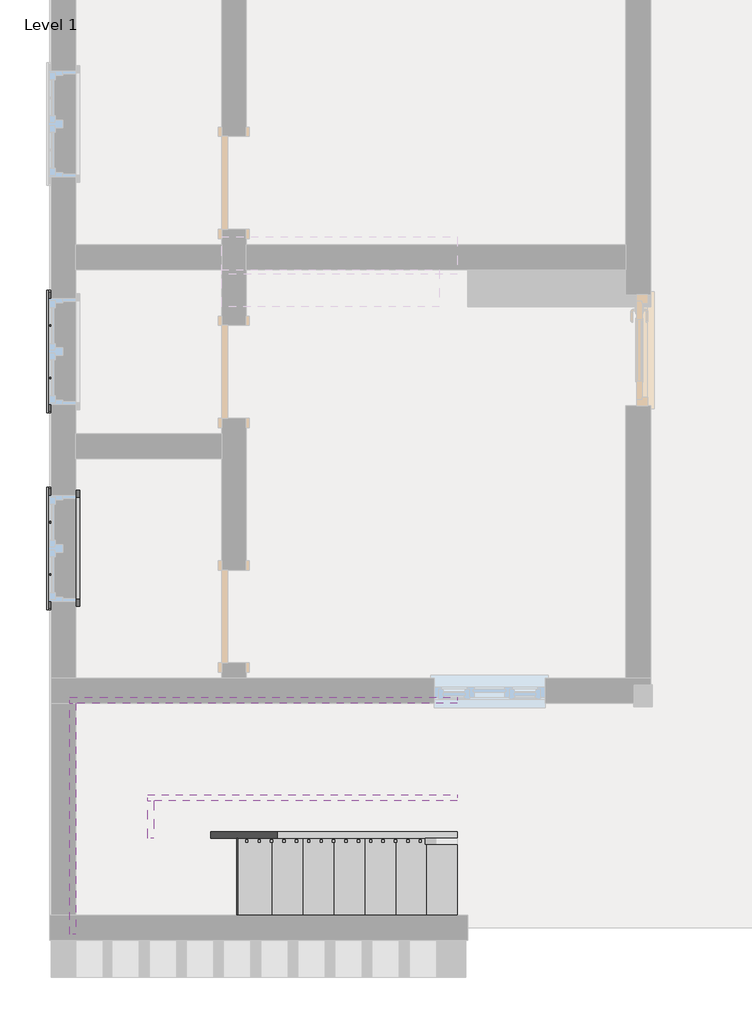
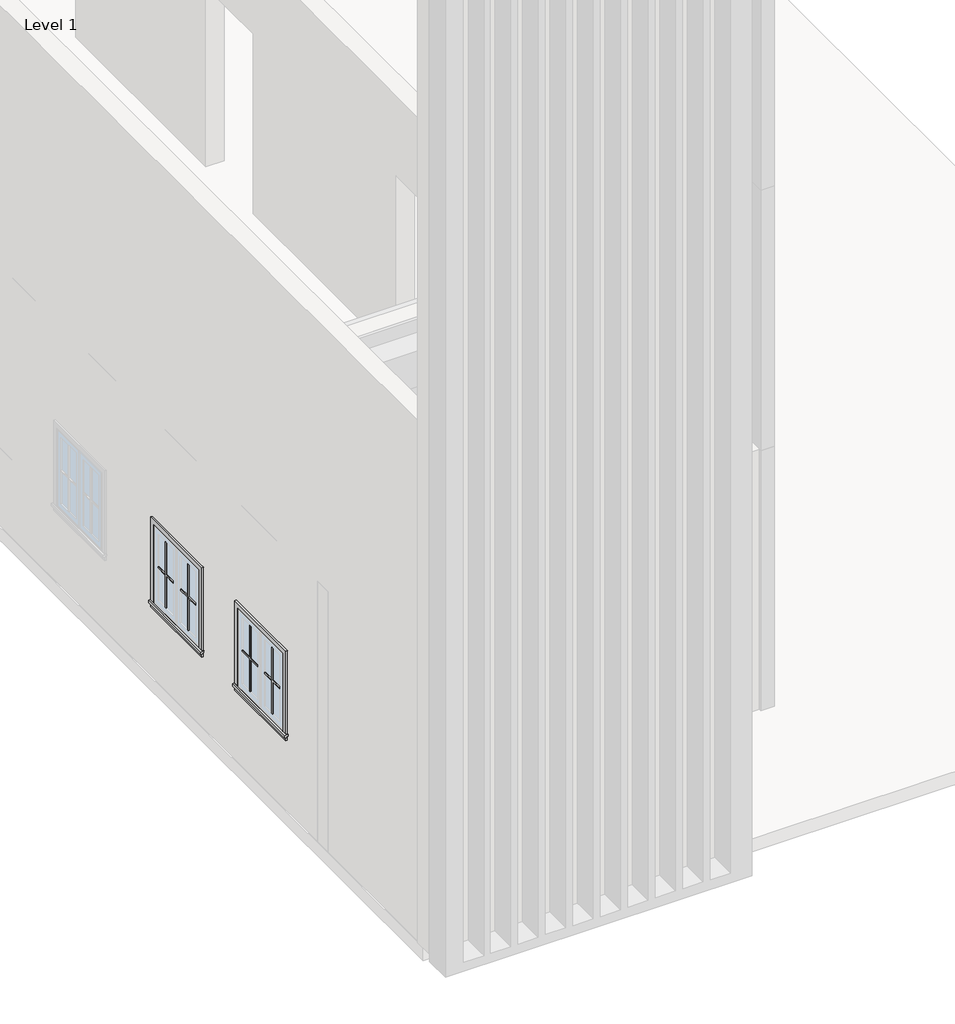
# One storey, part 3 of 4: 7 proxies, 6 members, 1 railing, 1 stair flight.
"""IFC4 building model written with IfcOpenShell, lengths in millimetres."""

from ifc_helpers import new_model, si_unit, frame, origin, place, context, project, spatial, polyline, outline, extrude, faceted_brep, transform, mapped, element, save
from components import muntin_pattern_2x2_muntin_pattern_2x2_b3fe6957, muntin_pattern_2x2_muntin_pattern_2x2_3e0ecaf2, trim_window_exterior_flat_with_sill_41619996, trim_window_interior_flat_picture_frame_51c85655, stair_flight_05893867

model = new_model("IFC4")

# Units and contexts
model_context = context("Model", 3, world=origin())
ifc_project = project(units=[si_unit("LENGTHUNIT", "METRE", prefix="MILLI")], contexts=[model_context])

# Site, building, storey
site = spatial("IfcSite", under=ifc_project)
building = spatial("IfcBuilding", under=site)
storey = spatial("IfcBuildingStorey", under=building, Name="Level 1", Elevation=0.0)

# Proxies
placement = place(None, origin())
muntin_pattern_2x2_muntin_pattern_2x2_shape = muntin_pattern_2x2_muntin_pattern_2x2_b3fe6957(model_context)
element("IfcBuildingElementProxy", 1, Name="Muntin Pattern_2x2 : Muntin Pattern_2x2", ObjectType="Muntin Pattern_2x2 : Muntin Pattern_2x2", at=placement, inside=storey, context=model_context, shape_type="MappedRepresentation", body=[
    mapped(muntin_pattern_2x2_muntin_pattern_2x2_shape, transform((-6438.8858866, -3658.1725272, 984.25), x_axis=(0.0, 1.0, 0.0), y_axis=(-1.0, 0.0, 0.0), z_axis=(0.0, 0.0, 1.0))),
])
element("IfcBuildingElementProxy", 2, Name="Muntin Pattern_2x2 : Muntin Pattern_2x2", ObjectType="Muntin Pattern_2x2 : Muntin Pattern_2x2", at=placement, inside=storey, context=model_context, shape_type="MappedRepresentation", body=[
    mapped(muntin_pattern_2x2_muntin_pattern_2x2_shape, transform((-6438.8858866, -5271.0725272, 984.25), x_axis=(0.0, 1.0, 0.0), y_axis=(-1.0, 0.0, 0.0), z_axis=(0.0, 0.0, 1.0))),
])
muntin_pattern_2x2_muntin_pattern_2x2_2_shape = muntin_pattern_2x2_muntin_pattern_2x2_3e0ecaf2(model_context)
element("IfcBuildingElementProxy", 3, Name="Muntin Pattern_2x2 : Muntin Pattern_2x2", ObjectType="Muntin Pattern_2x2 : Muntin Pattern_2x2", at=placement, inside=storey, context=model_context, shape_type="MappedRepresentation", body=[
    mapped(muntin_pattern_2x2_muntin_pattern_2x2_2_shape, transform((-6438.8858866, -3229.5475272, 984.25), x_axis=(0.0, -1.0, 0.0), y_axis=(1.0, 0.0, 0.0), z_axis=(0.0, 0.0, 1.0))),
])
element("IfcBuildingElementProxy", 4, Name="Muntin Pattern_2x2 : Muntin Pattern_2x2", ObjectType="Muntin Pattern_2x2 : Muntin Pattern_2x2", at=placement, inside=storey, context=model_context, shape_type="MappedRepresentation", body=[
    mapped(muntin_pattern_2x2_muntin_pattern_2x2_2_shape, transform((-6438.8858866, -4842.4475272, 984.25), x_axis=(0.0, -1.0, 0.0), y_axis=(1.0, 0.0, 0.0), z_axis=(0.0, 0.0, 1.0))),
])
trim_window_exterior_flat_with_sill_shape = trim_window_exterior_flat_with_sill_41619996(model_context)
element("IfcBuildingElementProxy", 5, Name="Trim-Window-Exterior-Flat : with Sill", ObjectType="Trim-Window-Exterior-Flat : with Sill", at=placement, inside=storey, context=model_context, shape_type="MappedRepresentation", body=[
    mapped(trim_window_exterior_flat_with_sill_shape, transform((-6448.4108866, -3443.8600272, 1828.8), x_axis=(0.0, -1.0, 0.0), y_axis=(0.0, 0.0, 1.0), z_axis=(-1.0, 0.0, 0.0))),
])
element("IfcBuildingElementProxy", 6, Name="Trim-Window-Exterior-Flat : with Sill", ObjectType="Trim-Window-Exterior-Flat : with Sill", at=placement, inside=storey, context=model_context, shape_type="MappedRepresentation", body=[
    mapped(trim_window_exterior_flat_with_sill_shape, transform((-6448.4108866, -5056.7600272, 1828.8), x_axis=(0.0, -1.0, 0.0), y_axis=(0.0, 0.0, 1.0), z_axis=(-1.0, 0.0, 0.0))),
])
trim_window_interior_flat_picture_frame_shape = trim_window_interior_flat_picture_frame_51c85655(model_context)
element("IfcBuildingElementProxy", 7, Name="Trim-Window-Interior-Flat : Picture Frame", ObjectType="Trim-Window-Interior-Flat : Picture Frame", at=placement, inside=storey, context=model_context, shape_type="MappedRepresentation", body=[
    mapped(trim_window_interior_flat_picture_frame_shape, transform((-6245.2108866, -5056.7600272, 1828.8), x_axis=(0.0, 1.0, 0.0), y_axis=(0.0, 0.0, 1.0), z_axis=(1.0, 0.0, 0.0))),
])

# Members
element("IfcMember", 8, ObjectType="Stringer - 2\" Width", at=placement, inside=storey, context=model_context, shape_type="SweptSolid", body=[
    extrude(outline(polyline([(0.0, -3117.2664982), (218.0398409, -3117.2664982), (1938.8666667, -5698.5067368), (1938.8666667, -6245.2108866), (1937.0120902, -6245.2108866), (0.0, -3339.6927512), (0.0, -3117.2664982)])), frame((0.0, -8219.0600272, 0.0), z_axis=(0.0, 1.0, 0.0), x_axis=(0.0, 0.0, 1.0)), (0.0, 0.0, 1.0), 50.8),
])
element("IfcMember", 9, ObjectType="Stringer - 2\" Width", at=placement, inside=storey, context=model_context, shape_type="SweptSolid", body=[
    extrude(outline(polyline([(-6245.2108866, -8219.0600272), (-6296.0108866, -8219.0600272), (-6296.0108866, -6326.7600272), (-6245.2108866, -6326.7600272), (-6245.2108866, -8219.0600272)])), frame((0.0, 0.0, 1634.0666667), z_axis=(0.0, 0.0, 1.0), x_axis=(1.0, 0.0, 0.0)), (0.0, 0.0, 1.0), 304.8),
])
element("IfcMember", 10, ObjectType="Stringer - 2\" Width", at=placement, inside=storey, context=model_context, shape_type="SweptSolid", body=[
    extrude(outline(polyline([(1695.0229713, -6296.0108866), (1634.0666667, -6296.0108866), (1634.0666667, -5800.9959317), (3224.4248495, -3117.2664982), (3578.7233496, -3117.2664982), (1695.0229713, -6296.0108866)])), frame((0.0, -6326.7600272, 0.0), z_axis=(0.0, 1.0, 0.0), x_axis=(0.0, 0.0, 1.0)), (0.0, 0.0, 1.0), 50.8),
])
element("IfcMember", 11, ObjectType="Stringer - 2\" Width", at=placement, inside=storey, context=model_context, shape_type="SweptSolid", body=[
    extrude(outline(polyline([(0.0, -3117.2664982), (218.0398409, -3117.2664982), (1877.5065076, -5606.4664982), (1511.182498, -5606.4664982), (0.0, -3339.6927512), (0.0, -3117.2664982)])), frame((0.0, -7431.6600272, 0.0), z_axis=(0.0, 1.0, 0.0), x_axis=(0.0, 0.0, 1.0)), (0.0, 0.0, 1.0), 50.8),
])
element("IfcMember", 12, ObjectType="Stringer - 2\" Width", at=placement, inside=storey, context=model_context, shape_type="SweptSolid", body=[
    extrude(outline(polyline([(-5606.4664982, -7431.6600272), (-5657.2664982, -7431.6600272), (-5657.2664982, -7126.8600272), (-5606.4664982, -7126.8600272), (-5606.4664982, -7431.6600272)])), frame((0.0, 0.0, 1634.0666667), z_axis=(0.0, 0.0, 1.0), x_axis=(1.0, 0.0, 0.0)), (0.0, 0.0, 1.0), 304.8),
])
element("IfcMember", 13, ObjectType="Stringer - 2\" Width", at=placement, inside=storey, context=model_context, shape_type="SweptSolid", body=[
    extrude(outline(polyline([(2073.5381644, -5657.2664982), (1719.2396643, -5657.2664982), (3224.4248495, -3117.2664982), (3578.7233496, -3117.2664982), (2073.5381644, -5657.2664982)])), frame((0.0, -7126.8600272, 0.0), z_axis=(0.0, 1.0, 0.0), x_axis=(0.0, 0.0, 1.0)), (0.0, 0.0, 1.0), 50.8),
])

# Railing
element("IfcRailing", 14, ObjectType="Handrail - Rectangular", at=placement, inside=storey, context=model_context, shape_type="SolidModel", body=[
    faceted_brep([(-3117.2664982, -8168.2600272, 1083.7333333), (-3117.2664982, -8168.2600272, 1022.6793317), (-3117.2664982, -8117.4600272, 1022.6793317), (-3117.2664982, -8117.4600272, 1083.7333333), (-5657.2664982, -8168.2600272, 2777.0666667), (-5672.6475006, -8168.2600272, 2726.2666667), (-5672.6475006, -8117.4600272, 2726.2666667), (-5657.2664982, -8117.4600272, 2777.0666667), (-6245.2108866, -8168.2600272, 2777.0666667), (-6245.2108866, -8168.2600272, 2726.2666667), (-6194.4108866, -8117.4600272, 2726.2666667), (-6194.4108866, -8117.4600272, 2777.0666667), (-6245.2108866, -6326.7600272, 2777.0666667), (-6245.2108866, -6326.7600272, 2726.2666667), (-6194.4108866, -6377.5600272, 2726.2666667), (-6194.4108866, -6377.5600272, 2777.0666667), (-5939.4887204, -6326.7600272, 2777.0666667), (-5925.417935, -6326.7600272, 2726.2666667), (-5925.417935, -6377.5600272, 2726.2666667), (-5939.4887204, -6377.5600272, 2777.0666667), (-3117.2664982, -6326.7600272, 4470.4), (-3117.2664982, -6377.5600272, 4470.4), (-3117.2664982, -6377.5600272, 4411.1575287), (-3117.2664982, -6326.7600272, 4411.1575287)], [[[0, 1, 2, 3]], [[1, 0, 4, 5]], [[2, 1, 5, 6]], [[3, 2, 6, 7]], [[0, 3, 7, 4]], [[5, 4, 8, 9]], [[6, 5, 9, 10]], [[7, 6, 10, 11]], [[4, 7, 11, 8]], [[9, 8, 12, 13]], [[10, 9, 13, 14]], [[11, 10, 14, 15]], [[8, 11, 15, 12]], [[13, 12, 16, 17]], [[14, 13, 17, 18]], [[15, 14, 18, 19]], [[12, 15, 19, 16]], [[20, 21, 22, 23]], [[17, 16, 20, 23]], [[18, 17, 23, 22]], [[19, 18, 22, 21]], [[16, 19, 21, 20]]]),
    extrude(outline(polyline([(4372.7158957, -3181.3358866), (3386.6666667, -3181.3358866), (3386.6666667, -3162.2858866), (4384.1458957, -3162.2858866), (4372.7158957, -3181.3358866)])), frame((0.0, -6361.6850272, 0.0), z_axis=(0.0, 1.0, 0.0), x_axis=(0.0, 0.0, 1.0)), (0.0, 0.0, 1.0), 19.05),
    extrude(outline(polyline([(4311.7558957, -3282.9358866), (3386.6666667, -3282.9358866), (3386.6666667, -3263.8858866), (4323.1858957, -3263.8858866), (4311.7558957, -3282.9358866)])), frame((0.0, -6361.6850272, 0.0), z_axis=(0.0, 1.0, 0.0), x_axis=(0.0, 0.0, 1.0)), (0.0, 0.0, 1.0), 19.05),
    extrude(outline(polyline([(4250.7958957, -3384.5358866), (3217.3333333, -3384.5358866), (3217.3333333, -3365.4858866), (4262.2258957, -3365.4858866), (4250.7958957, -3384.5358866)])), frame((0.0, -6361.6850272, 0.0), z_axis=(0.0, 1.0, 0.0), x_axis=(0.0, 0.0, 1.0)), (0.0, 0.0, 1.0), 19.05),
    extrude(outline(polyline([(4189.8358957, -3486.1358866), (3217.3333333, -3486.1358866), (3217.3333333, -3467.0858866), (4201.2658957, -3467.0858866), (4189.8358957, -3486.1358866)])), frame((0.0, -6361.6850272, 0.0), z_axis=(0.0, 1.0, 0.0), x_axis=(0.0, 0.0, 1.0)), (0.0, 0.0, 1.0), 19.05),
    extrude(outline(polyline([(4128.8758957, -3587.7358866), (3217.3333333, -3587.7358866), (3217.3333333, -3568.6858866), (4140.3058957, -3568.6858866), (4128.8758957, -3587.7358866)])), frame((0.0, -6361.6850272, 0.0), z_axis=(0.0, 1.0, 0.0), x_axis=(0.0, 0.0, 1.0)), (0.0, 0.0, 1.0), 19.05),
    extrude(outline(polyline([(4067.9158957, -3689.3358866), (3048.0, -3689.3358866), (3048.0, -3670.2858866), (4079.3458957, -3670.2858866), (4067.9158957, -3689.3358866)])), frame((0.0, -6361.6850272, 0.0), z_axis=(0.0, 1.0, 0.0), x_axis=(0.0, 0.0, 1.0)), (0.0, 0.0, 1.0), 19.05),
    extrude(outline(polyline([(4006.9558957, -3790.9358866), (3048.0, -3790.9358866), (3048.0, -3771.8858866), (4018.3858957, -3771.8858866), (4006.9558957, -3790.9358866)])), frame((0.0, -6361.6850272, 0.0), z_axis=(0.0, 1.0, 0.0), x_axis=(0.0, 0.0, 1.0)), (0.0, 0.0, 1.0), 19.05),
    extrude(outline(polyline([(3945.9958957, -3892.5358866), (3048.0, -3892.5358866), (3048.0, -3873.4858866), (3957.4258957, -3873.4858866), (3945.9958957, -3892.5358866)])), frame((0.0, -6361.6850272, 0.0), z_axis=(0.0, 1.0, 0.0), x_axis=(0.0, 0.0, 1.0)), (0.0, 0.0, 1.0), 19.05),
    extrude(outline(polyline([(3885.0358957, -3994.1358866), (3048.0, -3994.1358866), (3048.0, -3975.0858866), (3896.4658957, -3975.0858866), (3885.0358957, -3994.1358866)])), frame((0.0, -6361.6850272, 0.0), z_axis=(0.0, 1.0, 0.0), x_axis=(0.0, 0.0, 1.0)), (0.0, 0.0, 1.0), 19.05),
    extrude(outline(polyline([(3824.0758957, -4095.7358866), (3048.0, -4095.7358866), (3048.0, -4076.6858866), (3835.5058957, -4076.6858866), (3824.0758957, -4095.7358866)])), frame((0.0, -6361.6850272, 0.0), z_axis=(0.0, 1.0, 0.0), x_axis=(0.0, 0.0, 1.0)), (0.0, 0.0, 1.0), 19.05),
    extrude(outline(polyline([(3763.1158957, -4197.3358866), (2878.6666667, -4197.3358866), (2878.6666667, -4178.2858866), (3774.5458957, -4178.2858866), (3763.1158957, -4197.3358866)])), frame((0.0, -6361.6850272, 0.0), z_axis=(0.0, 1.0, 0.0), x_axis=(0.0, 0.0, 1.0)), (0.0, 0.0, 1.0), 19.05),
    extrude(outline(polyline([(3702.1558957, -4298.9358866), (2878.6666667, -4298.9358866), (2878.6666667, -4279.8858866), (3713.5858957, -4279.8858866), (3702.1558957, -4298.9358866)])), frame((0.0, -6361.6850272, 0.0), z_axis=(0.0, 1.0, 0.0), x_axis=(0.0, 0.0, 1.0)), (0.0, 0.0, 1.0), 19.05),
    extrude(outline(polyline([(3641.1958957, -4400.5358866), (2709.3333333, -4400.5358866), (2709.3333333, -4381.4858866), (3652.6258957, -4381.4858866), (3641.1958957, -4400.5358866)])), frame((0.0, -6361.6850272, 0.0), z_axis=(0.0, 1.0, 0.0), x_axis=(0.0, 0.0, 1.0)), (0.0, 0.0, 1.0), 19.05),
    extrude(outline(polyline([(3580.2358957, -4502.1358866), (2709.3333333, -4502.1358866), (2709.3333333, -4483.0858866), (3591.6658957, -4483.0858866), (3580.2358957, -4502.1358866)])), frame((0.0, -6361.6850272, 0.0), z_axis=(0.0, 1.0, 0.0), x_axis=(0.0, 0.0, 1.0)), (0.0, 0.0, 1.0), 19.05),
    extrude(outline(polyline([(3519.2758957, -4603.7358866), (2709.3333333, -4603.7358866), (2709.3333333, -4584.6858866), (3530.7058957, -4584.6858866), (3519.2758957, -4603.7358866)])), frame((0.0, -6361.6850272, 0.0), z_axis=(0.0, 1.0, 0.0), x_axis=(0.0, 0.0, 1.0)), (0.0, 0.0, 1.0), 19.05),
    extrude(outline(polyline([(3458.3158957, -4705.3358866), (2540.0, -4705.3358866), (2540.0, -4686.2858866), (3469.7458957, -4686.2858866), (3458.3158957, -4705.3358866)])), frame((0.0, -6361.6850272, 0.0), z_axis=(0.0, 1.0, 0.0), x_axis=(0.0, 0.0, 1.0)), (0.0, 0.0, 1.0), 19.05),
    extrude(outline(polyline([(3397.3558957, -4806.9358866), (2540.0, -4806.9358866), (2540.0, -4787.8858866), (3408.7858957, -4787.8858866), (3397.3558957, -4806.9358866)])), frame((0.0, -6361.6850272, 0.0), z_axis=(0.0, 1.0, 0.0), x_axis=(0.0, 0.0, 1.0)), (0.0, 0.0, 1.0), 19.05),
    extrude(outline(polyline([(3336.3958957, -4908.5358866), (2370.6666667, -4908.5358866), (2370.6666667, -4889.4858866), (3347.8258957, -4889.4858866), (3336.3958957, -4908.5358866)])), frame((0.0, -6361.6850272, 0.0), z_axis=(0.0, 1.0, 0.0), x_axis=(0.0, 0.0, 1.0)), (0.0, 0.0, 1.0), 19.05),
    extrude(outline(polyline([(3275.4358957, -5010.1358866), (2370.6666667, -5010.1358866), (2370.6666667, -4991.0858866), (3286.8658957, -4991.0858866), (3275.4358957, -5010.1358866)])), frame((0.0, -6361.6850272, 0.0), z_axis=(0.0, 1.0, 0.0), x_axis=(0.0, 0.0, 1.0)), (0.0, 0.0, 1.0), 19.05),
    extrude(outline(polyline([(3214.4758957, -5111.7358866), (2370.6666667, -5111.7358866), (2370.6666667, -5092.6858866), (3225.9058957, -5092.6858866), (3214.4758957, -5111.7358866)])), frame((0.0, -6361.6850272, 0.0), z_axis=(0.0, 1.0, 0.0), x_axis=(0.0, 0.0, 1.0)), (0.0, 0.0, 1.0), 19.05),
    extrude(outline(polyline([(3153.5158957, -5213.3358866), (2201.3333333, -5213.3358866), (2201.3333333, -5194.2858866), (3164.9458957, -5194.2858866), (3153.5158957, -5213.3358866)])), frame((0.0, -6361.6850272, 0.0), z_axis=(0.0, 1.0, 0.0), x_axis=(0.0, 0.0, 1.0)), (0.0, 0.0, 1.0), 19.05),
    extrude(outline(polyline([(3092.5558957, -5314.9358866), (2201.3333333, -5314.9358866), (2201.3333333, -5295.8858866), (3103.9858957, -5295.8858866), (3092.5558957, -5314.9358866)])), frame((0.0, -6361.6850272, 0.0), z_axis=(0.0, 1.0, 0.0), x_axis=(0.0, 0.0, 1.0)), (0.0, 0.0, 1.0), 19.05),
    extrude(outline(polyline([(3031.5958957, -5416.5358866), (2032.0, -5416.5358866), (2032.0, -5397.4858866), (3043.0258957, -5397.4858866), (3031.5958957, -5416.5358866)])), frame((0.0, -6361.6850272, 0.0), z_axis=(0.0, 1.0, 0.0), x_axis=(0.0, 0.0, 1.0)), (0.0, 0.0, 1.0), 19.05),
    extrude(outline(polyline([(2970.6358957, -5518.1358866), (2032.0, -5518.1358866), (2032.0, -5499.0858866), (2982.0658957, -5499.0858866), (2970.6358957, -5518.1358866)])), frame((0.0, -6361.6850272, 0.0), z_axis=(0.0, 1.0, 0.0), x_axis=(0.0, 0.0, 1.0)), (0.0, 0.0, 1.0), 19.05),
    extrude(outline(polyline([(2909.6758957, -5619.7358866), (2032.0, -5619.7358866), (2032.0, -5600.6858866), (2921.1058957, -5600.6858866), (2909.6758957, -5619.7358866)])), frame((0.0, -6361.6850272, 0.0), z_axis=(0.0, 1.0, 0.0), x_axis=(0.0, 0.0, 1.0)), (0.0, 0.0, 1.0), 19.05),
    extrude(outline(polyline([(2848.7158957, -5721.3358866), (1862.6666667, -5721.3358866), (1862.6666667, -5702.2858866), (2860.1458957, -5702.2858866), (2848.7158957, -5721.3358866)])), frame((0.0, -6361.6850272, 0.0), z_axis=(0.0, 1.0, 0.0), x_axis=(0.0, 0.0, 1.0)), (0.0, 0.0, 1.0), 19.05),
    extrude(outline(polyline([(2787.7558957, -5822.9358866), (1862.6666667, -5822.9358866), (1862.6666667, -5803.8858866), (2799.1858957, -5803.8858866), (2787.7558957, -5822.9358866)])), frame((0.0, -6361.6850272, 0.0), z_axis=(0.0, 1.0, 0.0), x_axis=(0.0, 0.0, 1.0)), (0.0, 0.0, 1.0), 19.05),
    extrude(outline(polyline([(2726.7958957, -5924.5358866), (1862.6666667, -5924.5358866), (1862.6666667, -5905.4858866), (2738.2258957, -5905.4858866), (2726.7958957, -5924.5358866)])), frame((0.0, -6361.6850272, 0.0), z_axis=(0.0, 1.0, 0.0), x_axis=(0.0, 0.0, 1.0)), (0.0, 0.0, 1.0), 19.05),
    extrude(outline(polyline([(-6026.1358866, -6342.6350272), (-6007.0858866, -6342.6350272), (-6007.0858866, -6361.6850272), (-6026.1358866, -6361.6850272), (-6026.1358866, -6342.6350272)])), frame((0.0, 0.0, 1862.6666667), z_axis=(0.0, 0.0, 1.0), x_axis=(1.0, 0.0, 0.0)), (0.0, 0.0, 1.0), 863.6),
    extrude(outline(polyline([(-6127.7358866, -6342.6350272), (-6108.6858866, -6342.6350272), (-6108.6858866, -6361.6850272), (-6127.7358866, -6361.6850272), (-6127.7358866, -6342.6350272)])), frame((0.0, 0.0, 1862.6666667), z_axis=(0.0, 0.0, 1.0), x_axis=(1.0, 0.0, 0.0)), (0.0, 0.0, 1.0), 863.6),
    extrude(outline(polyline([(-6229.3358866, -6425.1850272), (-6229.3358866, -6406.1350272), (-6210.2858866, -6406.1350272), (-6210.2858866, -6425.1850272), (-6229.3358866, -6425.1850272)])), frame((0.0, 0.0, 1862.6666667), z_axis=(0.0, 0.0, 1.0), x_axis=(1.0, 0.0, 0.0)), (0.0, 0.0, 1.0), 863.6),
    extrude(outline(polyline([(-6229.3358866, -6526.7850272), (-6229.3358866, -6507.7350272), (-6210.2858866, -6507.7350272), (-6210.2858866, -6526.7850272), (-6229.3358866, -6526.7850272)])), frame((0.0, 0.0, 1862.6666667), z_axis=(0.0, 0.0, 1.0), x_axis=(1.0, 0.0, 0.0)), (0.0, 0.0, 1.0), 863.6),
    extrude(outline(polyline([(-6229.3358866, -6628.3850272), (-6229.3358866, -6609.3350272), (-6210.2858866, -6609.3350272), (-6210.2858866, -6628.3850272), (-6229.3358866, -6628.3850272)])), frame((0.0, 0.0, 1862.6666667), z_axis=(0.0, 0.0, 1.0), x_axis=(1.0, 0.0, 0.0)), (0.0, 0.0, 1.0), 863.6),
    extrude(outline(polyline([(-6229.3358866, -6729.9850272), (-6229.3358866, -6710.9350272), (-6210.2858866, -6710.9350272), (-6210.2858866, -6729.9850272), (-6229.3358866, -6729.9850272)])), frame((0.0, 0.0, 1862.6666667), z_axis=(0.0, 0.0, 1.0), x_axis=(1.0, 0.0, 0.0)), (0.0, 0.0, 1.0), 863.6),
    extrude(outline(polyline([(-6229.3358866, -6831.5850272), (-6229.3358866, -6812.5350272), (-6210.2858866, -6812.5350272), (-6210.2858866, -6831.5850272), (-6229.3358866, -6831.5850272)])), frame((0.0, 0.0, 1862.6666667), z_axis=(0.0, 0.0, 1.0), x_axis=(1.0, 0.0, 0.0)), (0.0, 0.0, 1.0), 863.6),
    extrude(outline(polyline([(-6229.3358866, -6933.1850272), (-6229.3358866, -6914.1350272), (-6210.2858866, -6914.1350272), (-6210.2858866, -6933.1850272), (-6229.3358866, -6933.1850272)])), frame((0.0, 0.0, 1862.6666667), z_axis=(0.0, 0.0, 1.0), x_axis=(1.0, 0.0, 0.0)), (0.0, 0.0, 1.0), 863.6),
    extrude(outline(polyline([(-6229.3358866, -7034.7850272), (-6229.3358866, -7015.7350272), (-6210.2858866, -7015.7350272), (-6210.2858866, -7034.7850272), (-6229.3358866, -7034.7850272)])), frame((0.0, 0.0, 1862.6666667), z_axis=(0.0, 0.0, 1.0), x_axis=(1.0, 0.0, 0.0)), (0.0, 0.0, 1.0), 863.6),
    extrude(outline(polyline([(-6229.3358866, -7136.3850272), (-6229.3358866, -7117.3350272), (-6210.2858866, -7117.3350272), (-6210.2858866, -7136.3850272), (-6229.3358866, -7136.3850272)])), frame((0.0, 0.0, 1862.6666667), z_axis=(0.0, 0.0, 1.0), x_axis=(1.0, 0.0, 0.0)), (0.0, 0.0, 1.0), 863.6),
    extrude(outline(polyline([(-6229.3358866, -7237.9850272), (-6229.3358866, -7218.9350272), (-6210.2858866, -7218.9350272), (-6210.2858866, -7237.9850272), (-6229.3358866, -7237.9850272)])), frame((0.0, 0.0, 1862.6666667), z_axis=(0.0, 0.0, 1.0), x_axis=(1.0, 0.0, 0.0)), (0.0, 0.0, 1.0), 863.6),
    extrude(outline(polyline([(-6229.3358866, -7339.5850272), (-6229.3358866, -7320.5350272), (-6210.2858866, -7320.5350272), (-6210.2858866, -7339.5850272), (-6229.3358866, -7339.5850272)])), frame((0.0, 0.0, 1862.6666667), z_axis=(0.0, 0.0, 1.0), x_axis=(1.0, 0.0, 0.0)), (0.0, 0.0, 1.0), 863.6),
    extrude(outline(polyline([(-6229.3358866, -7441.1850272), (-6229.3358866, -7422.1350272), (-6210.2858866, -7422.1350272), (-6210.2858866, -7441.1850272), (-6229.3358866, -7441.1850272)])), frame((0.0, 0.0, 1862.6666667), z_axis=(0.0, 0.0, 1.0), x_axis=(1.0, 0.0, 0.0)), (0.0, 0.0, 1.0), 863.6),
    extrude(outline(polyline([(-6229.3358866, -7542.7850272), (-6229.3358866, -7523.7350272), (-6210.2858866, -7523.7350272), (-6210.2858866, -7542.7850272), (-6229.3358866, -7542.7850272)])), frame((0.0, 0.0, 1862.6666667), z_axis=(0.0, 0.0, 1.0), x_axis=(1.0, 0.0, 0.0)), (0.0, 0.0, 1.0), 863.6),
    extrude(outline(polyline([(-6229.3358866, -7644.3850272), (-6229.3358866, -7625.3350272), (-6210.2858866, -7625.3350272), (-6210.2858866, -7644.3850272), (-6229.3358866, -7644.3850272)])), frame((0.0, 0.0, 1862.6666667), z_axis=(0.0, 0.0, 1.0), x_axis=(1.0, 0.0, 0.0)), (0.0, 0.0, 1.0), 863.6),
    extrude(outline(polyline([(-6229.3358866, -7745.9850272), (-6229.3358866, -7726.9350272), (-6210.2858866, -7726.9350272), (-6210.2858866, -7745.9850272), (-6229.3358866, -7745.9850272)])), frame((0.0, 0.0, 1862.6666667), z_axis=(0.0, 0.0, 1.0), x_axis=(1.0, 0.0, 0.0)), (0.0, 0.0, 1.0), 863.6),
    extrude(outline(polyline([(-6229.3358866, -7847.5850272), (-6229.3358866, -7828.5350272), (-6210.2858866, -7828.5350272), (-6210.2858866, -7847.5850272), (-6229.3358866, -7847.5850272)])), frame((0.0, 0.0, 1862.6666667), z_axis=(0.0, 0.0, 1.0), x_axis=(1.0, 0.0, 0.0)), (0.0, 0.0, 1.0), 863.6),
    extrude(outline(polyline([(-6229.3358866, -7949.1850272), (-6229.3358866, -7930.1350272), (-6210.2858866, -7930.1350272), (-6210.2858866, -7949.1850272), (-6229.3358866, -7949.1850272)])), frame((0.0, 0.0, 1862.6666667), z_axis=(0.0, 0.0, 1.0), x_axis=(1.0, 0.0, 0.0)), (0.0, 0.0, 1.0), 863.6),
    extrude(outline(polyline([(-6229.3358866, -8050.7850272), (-6229.3358866, -8031.7350272), (-6210.2858866, -8031.7350272), (-6210.2858866, -8050.7850272), (-6229.3358866, -8050.7850272)])), frame((0.0, 0.0, 1862.6666667), z_axis=(0.0, 0.0, 1.0), x_axis=(1.0, 0.0, 0.0)), (0.0, 0.0, 1.0), 863.6),
    extrude(outline(polyline([(-6155.7414982, -8152.3850272), (-6174.7914982, -8152.3850272), (-6174.7914982, -8133.3350272), (-6155.7414982, -8133.3350272), (-6155.7414982, -8152.3850272)])), frame((0.0, 0.0, 1862.6666667), z_axis=(0.0, 0.0, 1.0), x_axis=(1.0, 0.0, 0.0)), (0.0, 0.0, 1.0), 863.6),
    extrude(outline(polyline([(-6054.1414982, -8152.3850272), (-6073.1914982, -8152.3850272), (-6073.1914982, -8133.3350272), (-6054.1414982, -8133.3350272), (-6054.1414982, -8152.3850272)])), frame((0.0, 0.0, 1862.6666667), z_axis=(0.0, 0.0, 1.0), x_axis=(1.0, 0.0, 0.0)), (0.0, 0.0, 1.0), 863.6),
    extrude(outline(polyline([(-5952.5414982, -8152.3850272), (-5971.5914982, -8152.3850272), (-5971.5914982, -8133.3350272), (-5952.5414982, -8133.3350272), (-5952.5414982, -8152.3850272)])), frame((0.0, 0.0, 1862.6666667), z_axis=(0.0, 0.0, 1.0), x_axis=(1.0, 0.0, 0.0)), (0.0, 0.0, 1.0), 863.6),
    extrude(outline(polyline([(-5850.9414982, -8152.3850272), (-5869.9914982, -8152.3850272), (-5869.9914982, -8133.3350272), (-5850.9414982, -8133.3350272), (-5850.9414982, -8152.3850272)])), frame((0.0, 0.0, 1862.6666667), z_axis=(0.0, 0.0, 1.0), x_axis=(1.0, 0.0, 0.0)), (0.0, 0.0, 1.0), 863.6),
    extrude(outline(polyline([(-5749.3414982, -8152.3850272), (-5768.3914982, -8152.3850272), (-5768.3914982, -8133.3350272), (-5749.3414982, -8133.3350272), (-5749.3414982, -8152.3850272)])), frame((0.0, 0.0, 1862.6666667), z_axis=(0.0, 0.0, 1.0), x_axis=(1.0, 0.0, 0.0)), (0.0, 0.0, 1.0), 863.6),
    extrude(outline(polyline([(2722.3626651, -5666.7914982), (1862.6666667, -5666.7914982), (1862.6666667, -5647.7414982), (2709.6626651, -5647.7414982), (2722.3626651, -5666.7914982)])), frame((0.0, -8152.3850272, 0.0), z_axis=(0.0, 1.0, 0.0), x_axis=(0.0, 0.0, 1.0)), (0.0, 0.0, 1.0), 19.05),
    extrude(outline(polyline([(2654.6293317, -5565.1914982), (1693.3333333, -5565.1914982), (1693.3333333, -5546.1414982), (2641.9293317, -5546.1414982), (2654.6293317, -5565.1914982)])), frame((0.0, -8152.3850272, 0.0), z_axis=(0.0, 1.0, 0.0), x_axis=(0.0, 0.0, 1.0)), (0.0, 0.0, 1.0), 19.05),
    extrude(outline(polyline([(2586.8959984, -5463.5914982), (1693.3333333, -5463.5914982), (1693.3333333, -5444.5414982), (2574.1959984, -5444.5414982), (2586.8959984, -5463.5914982)])), frame((0.0, -8152.3850272, 0.0), z_axis=(0.0, 1.0, 0.0), x_axis=(0.0, 0.0, 1.0)), (0.0, 0.0, 1.0), 19.05),
    extrude(outline(polyline([(2519.1626651, -5361.9914982), (1524.0, -5361.9914982), (1524.0, -5342.9414982), (2506.4626651, -5342.9414982), (2519.1626651, -5361.9914982)])), frame((0.0, -8152.3850272, 0.0), z_axis=(0.0, 1.0, 0.0), x_axis=(0.0, 0.0, 1.0)), (0.0, 0.0, 1.0), 19.05),
    extrude(outline(polyline([(2451.4293317, -5260.3914982), (1524.0, -5260.3914982), (1524.0, -5241.3414982), (2438.7293317, -5241.3414982), (2451.4293317, -5260.3914982)])), frame((0.0, -8152.3850272, 0.0), z_axis=(0.0, 1.0, 0.0), x_axis=(0.0, 0.0, 1.0)), (0.0, 0.0, 1.0), 19.05),
    extrude(outline(polyline([(2383.6959984, -5158.7914982), (1524.0, -5158.7914982), (1524.0, -5139.7414982), (2370.9959984, -5139.7414982), (2383.6959984, -5158.7914982)])), frame((0.0, -8152.3850272, 0.0), z_axis=(0.0, 1.0, 0.0), x_axis=(0.0, 0.0, 1.0)), (0.0, 0.0, 1.0), 19.05),
    extrude(outline(polyline([(2315.9626651, -5057.1914982), (1354.6666667, -5057.1914982), (1354.6666667, -5038.1414982), (2303.2626651, -5038.1414982), (2315.9626651, -5057.1914982)])), frame((0.0, -8152.3850272, 0.0), z_axis=(0.0, 1.0, 0.0), x_axis=(0.0, 0.0, 1.0)), (0.0, 0.0, 1.0), 19.05),
    extrude(outline(polyline([(2248.2293317, -4955.5914982), (1354.6666667, -4955.5914982), (1354.6666667, -4936.5414982), (2235.5293317, -4936.5414982), (2248.2293317, -4955.5914982)])), frame((0.0, -8152.3850272, 0.0), z_axis=(0.0, 1.0, 0.0), x_axis=(0.0, 0.0, 1.0)), (0.0, 0.0, 1.0), 19.05),
    extrude(outline(polyline([(2180.4959984, -4853.9914982), (1185.3333333, -4853.9914982), (1185.3333333, -4834.9414982), (2167.7959984, -4834.9414982), (2180.4959984, -4853.9914982)])), frame((0.0, -8152.3850272, 0.0), z_axis=(0.0, 1.0, 0.0), x_axis=(0.0, 0.0, 1.0)), (0.0, 0.0, 1.0), 19.05),
    extrude(outline(polyline([(2112.7626651, -4752.3914982), (1185.3333333, -4752.3914982), (1185.3333333, -4733.3414982), (2100.0626651, -4733.3414982), (2112.7626651, -4752.3914982)])), frame((0.0, -8152.3850272, 0.0), z_axis=(0.0, 1.0, 0.0), x_axis=(0.0, 0.0, 1.0)), (0.0, 0.0, 1.0), 19.05),
    extrude(outline(polyline([(2045.0293317, -4650.7914982), (1185.3333333, -4650.7914982), (1185.3333333, -4631.7414982), (2032.3293317, -4631.7414982), (2045.0293317, -4650.7914982)])), frame((0.0, -8152.3850272, 0.0), z_axis=(0.0, 1.0, 0.0), x_axis=(0.0, 0.0, 1.0)), (0.0, 0.0, 1.0), 19.05),
    extrude(outline(polyline([(1977.2959984, -4549.1914982), (1016.0, -4549.1914982), (1016.0, -4530.1414982), (1964.5959984, -4530.1414982), (1977.2959984, -4549.1914982)])), frame((0.0, -8152.3850272, 0.0), z_axis=(0.0, 1.0, 0.0), x_axis=(0.0, 0.0, 1.0)), (0.0, 0.0, 1.0), 19.05),
    extrude(outline(polyline([(1909.5626651, -4447.5914982), (1016.0, -4447.5914982), (1016.0, -4428.5414982), (1896.8626651, -4428.5414982), (1909.5626651, -4447.5914982)])), frame((0.0, -8152.3850272, 0.0), z_axis=(0.0, 1.0, 0.0), x_axis=(0.0, 0.0, 1.0)), (0.0, 0.0, 1.0), 19.05),
    extrude(outline(polyline([(1841.8293317, -4345.9914982), (846.6666667, -4345.9914982), (846.6666667, -4326.9414982), (1829.1293317, -4326.9414982), (1841.8293317, -4345.9914982)])), frame((0.0, -8152.3850272, 0.0), z_axis=(0.0, 1.0, 0.0), x_axis=(0.0, 0.0, 1.0)), (0.0, 0.0, 1.0), 19.05),
    extrude(outline(polyline([(1774.0959984, -4244.3914982), (846.6666667, -4244.3914982), (846.6666667, -4225.3414982), (1761.3959984, -4225.3414982), (1774.0959984, -4244.3914982)])), frame((0.0, -8152.3850272, 0.0), z_axis=(0.0, 1.0, 0.0), x_axis=(0.0, 0.0, 1.0)), (0.0, 0.0, 1.0), 19.05),
    extrude(outline(polyline([(1706.3626651, -4142.7914982), (846.6666667, -4142.7914982), (846.6666667, -4123.7414982), (1693.6626651, -4123.7414982), (1706.3626651, -4142.7914982)])), frame((0.0, -8152.3850272, 0.0), z_axis=(0.0, 1.0, 0.0), x_axis=(0.0, 0.0, 1.0)), (0.0, 0.0, 1.0), 19.05),
    extrude(outline(polyline([(1638.6293317, -4041.1914982), (677.3333333, -4041.1914982), (677.3333333, -4022.1414982), (1625.9293317, -4022.1414982), (1638.6293317, -4041.1914982)])), frame((0.0, -8152.3850272, 0.0), z_axis=(0.0, 1.0, 0.0), x_axis=(0.0, 0.0, 1.0)), (0.0, 0.0, 1.0), 19.05),
    extrude(outline(polyline([(1570.8959984, -3939.5914982), (677.3333333, -3939.5914982), (677.3333333, -3920.5414982), (1558.1959984, -3920.5414982), (1570.8959984, -3939.5914982)])), frame((0.0, -8152.3850272, 0.0), z_axis=(0.0, 1.0, 0.0), x_axis=(0.0, 0.0, 1.0)), (0.0, 0.0, 1.0), 19.05),
    extrude(outline(polyline([(1503.1626651, -3837.9914982), (508.0, -3837.9914982), (508.0, -3818.9414982), (1490.4626651, -3818.9414982), (1503.1626651, -3837.9914982)])), frame((0.0, -8152.3850272, 0.0), z_axis=(0.0, 1.0, 0.0), x_axis=(0.0, 0.0, 1.0)), (0.0, 0.0, 1.0), 19.05),
    extrude(outline(polyline([(1435.4293317, -3736.3914982), (508.0, -3736.3914982), (508.0, -3717.3414982), (1422.7293317, -3717.3414982), (1435.4293317, -3736.3914982)])), frame((0.0, -8152.3850272, 0.0), z_axis=(0.0, 1.0, 0.0), x_axis=(0.0, 0.0, 1.0)), (0.0, 0.0, 1.0), 19.05),
    extrude(outline(polyline([(1367.6959984, -3634.7914982), (508.0, -3634.7914982), (508.0, -3615.7414982), (1354.9959984, -3615.7414982), (1367.6959984, -3634.7914982)])), frame((0.0, -8152.3850272, 0.0), z_axis=(0.0, 1.0, 0.0), x_axis=(0.0, 0.0, 1.0)), (0.0, 0.0, 1.0), 19.05),
    extrude(outline(polyline([(1299.9626651, -3533.1914982), (338.6666667, -3533.1914982), (338.6666667, -3514.1414982), (1287.2626651, -3514.1414982), (1299.9626651, -3533.1914982)])), frame((0.0, -8152.3850272, 0.0), z_axis=(0.0, 1.0, 0.0), x_axis=(0.0, 0.0, 1.0)), (0.0, 0.0, 1.0), 19.05),
    extrude(outline(polyline([(1232.2293317, -3431.5914982), (338.6666667, -3431.5914982), (338.6666667, -3412.5414982), (1219.5293317, -3412.5414982), (1232.2293317, -3431.5914982)])), frame((0.0, -8152.3850272, 0.0), z_axis=(0.0, 1.0, 0.0), x_axis=(0.0, 0.0, 1.0)), (0.0, 0.0, 1.0), 19.05),
    extrude(outline(polyline([(1164.4959984, -3329.9914982), (169.3333333, -3329.9914982), (169.3333333, -3310.9414982), (1151.7959984, -3310.9414982), (1164.4959984, -3329.9914982)])), frame((0.0, -8152.3850272, 0.0), z_axis=(0.0, 1.0, 0.0), x_axis=(0.0, 0.0, 1.0)), (0.0, 0.0, 1.0), 19.05),
    extrude(outline(polyline([(1096.7626651, -3228.3914982), (169.3333333, -3228.3914982), (169.3333333, -3209.3414982), (1084.0626651, -3209.3414982), (1096.7626651, -3228.3914982)])), frame((0.0, -8152.3850272, 0.0), z_axis=(0.0, 1.0, 0.0), x_axis=(0.0, 0.0, 1.0)), (0.0, 0.0, 1.0), 19.05),
    extrude(outline(polyline([(-6229.3358866, -6361.6850272), (-6229.3358866, -6342.6350272), (-6210.2858866, -6342.6350272), (-6210.2858866, -6361.6850272), (-6229.3358866, -6361.6850272)])), frame((0.0, 0.0, 1862.6666667), z_axis=(0.0, 0.0, 1.0), x_axis=(1.0, 0.0, 0.0)), (0.0, 0.0, 1.0), 863.6),
    extrude(outline(polyline([(-6210.2858866, -8152.3850272), (-6229.3358866, -8152.3850272), (-6229.3358866, -8133.3350272), (-6210.2858866, -8133.3350272), (-6210.2858866, -8152.3850272)])), frame((0.0, 0.0, 1862.6666667), z_axis=(0.0, 0.0, 1.0), x_axis=(1.0, 0.0, 0.0)), (0.0, 0.0, 1.0), 863.6),
    extrude(outline(polyline([(4399.7275287, -3136.3164982), (3386.6666667, -3136.3164982), (3386.6666667, -3117.2664982), (4411.1575287, -3117.2664982), (4399.7275287, -3136.3164982)])), frame((0.0, -6361.6850272, 0.0), z_axis=(0.0, 1.0, 0.0), x_axis=(0.0, 0.0, 1.0)), (0.0, 0.0, 1.0), 19.05),
    extrude(outline(polyline([(1035.3793317, -3136.3164982), (169.3333333, -3136.3164982), (169.3333333, -3117.2664982), (1022.6793317, -3117.2664982), (1035.3793317, -3136.3164982)])), frame((0.0, -8152.3850272, 0.0), z_axis=(0.0, 1.0, 0.0), x_axis=(0.0, 0.0, 1.0)), (0.0, 0.0, 1.0), 19.05),
])

# Stair flight
stair_flight_shape = stair_flight_05893867(model_context)
element("IfcStairFlight", 15, ObjectType="2\" Tread 1\" Nosing 1/4\" Riser", at=placement, inside=storey, context=model_context, shape_type="MappedRepresentation", body=[
    mapped(stair_flight_shape, transform((0.0, 0.0, 0.0), x_axis=(1.0, 0.0, 0.0), y_axis=(0.0, 1.0, 0.0), z_axis=(0.0, 0.0, 1.0))),
])

save(model, "model.ifc")

# Revit data of these elements
# Type "Muntin Pattern_2x2 : Muntin Pattern_2x2"
#   Width [instance default] = 4' - 0"
#   Thickness = 0' - 0 1/2"
#   Height [instance default] = 4' - 0"
#   Distance = 0' - 0 3/4"
#   Interior Material [instance default] = none
#   Exterior Material [instance default] = none
#   Default Elevation = 0
# Type "Trim-Window-Exterior-Flat : with Sill"
#   Trim Width = 0' - 2 1/4"
#   Trim Thickness_Picture Frame = 0' - 1 1/4"
#   Trim Thickness_with Sill = 0' - 0 3/4"
#   Sill Thickness = 0' - 1 1/4"
#   Opening Width [instance default] = 2' - 0"
#   Opening Height [instance default] = 3' - 0"
#   Default Elevation = 4' - 0"
#   Sill = yes
#   Picture Frame = no
#   Trim Material [instance default] = none
# Type "Trim-Window-Interior-Flat : Picture Frame"
#   Trim Thickness_Picture Frame = 0' - 1 1/4"
#   Trim Width = 0' - 2 1/4"
#   Trim Thickness_with Sill = 0' - 0 3/4"
#   Sill Thickness = 0' - 1 1/4"
#   Opening Width [instance default] = 2' - 0"
#   Opening Height [instance default] = 3' - 0"
#   Default Elevation = 4' - 0"
#   Sill = no
#   Picture Frame = yes
#   Trim Material [instance default] = none
# Type "Handrail - Rectangular"
#   Assembly Code = "C2010400"
#   built-in parameter 1008612 = 0.0416667 (stored number, unit not read)
#   built-in parameter 1008611 = 0.0416667 (stored number, unit not read)
#   built-in parameter 1008609 = 0.333333 (stored number, unit not read)
#   built-in parameter 1008604 = 0.166667 (stored number, unit not read)
#   built-in parameter 1008603 = 0.166667 (stored number, unit not read)
#   Railing Height = 3' - 0"
#   built-in parameter 1008630 = 2
#   built-in parameter 1008610 = 2
#   built-in parameter 1008618 = Baluster - Square : 3/4"
# Elements 1, 2, 3, 4 (IfcBuildingElementProxy, "Muntin Pattern_2x2 : Muntin Pattern_2x2")
#   Width = 0' - 11 5/8"
#   Height = 2' - 6 1/2"
#   Interior Material = Wood - Stained
#   Exterior Material = Clad - White
#   Phase Created = New Construction
#   Materials on its faces: "Clad - White", "Wood - Stained"
# Elements 5, 6 (IfcBuildingElementProxy, "Trim-Window-Exterior-Flat : with Sill")
#   Opening Width = 2' - 10"
#   Opening Height = 3' - 0"
#   Trim Material = Clad - White
#   Phase Created = New Construction
#   Materials on its faces: "Clad - White"
# Element 7 (IfcBuildingElementProxy, "Trim-Window-Interior-Flat : Picture Frame")
#   Opening Width = 2' - 10"
#   Opening Height = 3' - 0"
#   Trim Material = Wood - Stained
#   Phase Created = New Construction
#   Materials on its faces: "Wood - Stained"
# Elements 8, 9, 10, 11, 12, 13 (IfcMember, "Stringer - 2\" Width")
#   Phase Created = New Construction
# Element 14 (IfcRailing, "Handrail - Rectangular")
#   Phase Created = New Construction
# Element 15 (IfcStairFlight, "2\" Tread 1\" Nosing 1/4\" Riser")
#   Phase Created = New Construction
# Materials
#   "Clad - White": class "Wood", colour RGB 242 242 238, transparency 0, Cost = 0
#   "Wood - Stained": class "Wood", colour RGB 224 178 126, transparency 0, Cost = 0
